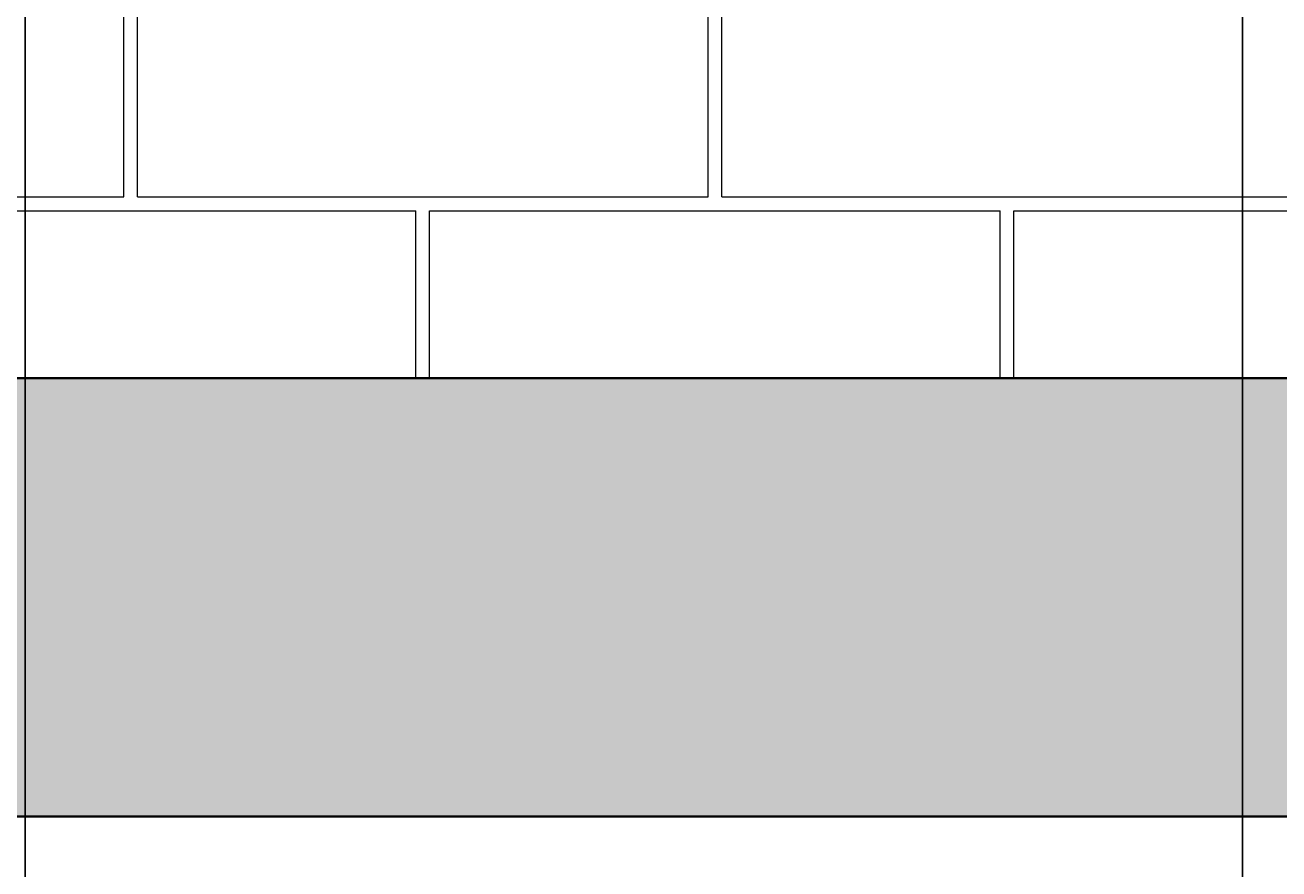
# Model space of a CAD drawing. Units: inches. Extents: x -301 to 715, y -607 to 364.
# Tile 131 of 141: x 310 to 362, y -510 to -475. Entities that reach past the tile are written whole.
import ezdxf

# ---------------------------------------------------------------- set-up
doc = ezdxf.new("R2010")
doc.units = ezdxf.units.IN
doc.header["$MEASUREMENT"] = 0
for name, color, linetype, lineweight in [('A-ANNO-DIMS', 2, 'Continuous', 18), ('A-ELEV', 220, 'Continuous', 30), ('A-ELEV-PATT', 4, 'Continuous', 13)]:
    doc.layers.add(name, color=color, linetype=linetype, lineweight=lineweight)
doc.styles.get("Standard").update_dxf_attribs({"font": 'arial.ttf'})
doc.dimstyles.get("Standard").update_dxf_attribs({"dimtxt": 0.18, "dimasz": 0.18, "dimexe": 0.18, "dimexo": 0.0625, "dimgap": 0.09, "dimtad": 0, "dimtih": 1, "dimtoh": 1, "dimdec": 1, "dimzin": 0, "dimdsep": 46, "dimlunit": 4, "dimtxsty": 'Standard', "dimcen": 0.09, "dimclrd": 3, "dimclre": 4, "dimclrt": 6, "dimadec": 0, "dimazin": 0, "dimtfac": 1, "dimtdec": 1, "dimtofl": 0, "dimtmove": 0, "dimatfit": 3, "dimfxl": 1, "dimtfill": 2, "dimtfillclr": 51, "dimtolj": 1, "dimtzin": 0, "dimarcsym": 0})

# ---------------------------------------------------------------- blocks, each defined once
blk = doc.blocks.new('*D195')
at = {"layer": 'A-ANNO-DIMS', "color": 4, "lineweight": -2, "transparency": 16777216}
for p, q in [((310.018, -441.615), (310.018, -606.789)), ((360.018, -441.615), (360.018, -606.789))]:
    blk.add_line(p, q, dxfattribs=at)
at = {"layer": 'A-ANNO-DIMS', "color": 3, "lineweight": -2, "transparency": 16777216}
for p, q in [((310.198, -606.609), (334.685, -606.609)), ((359.838, -606.609), (335.351, -606.609))]:
    blk.add_line(p, q, dxfattribs=at)
at = {"layer": 'A-ANNO-DIMS', "color": 3, "transparency": 16777216}
for points in [[(310.198, -606.579), (310.198, -606.639), (310.018, -606.609)], [(359.838, -606.579), (359.838, -606.639), (360.018, -606.609)]]:
    blk.add_solid(points, dxfattribs=at)
at = {"layer": 'Defpoints', "color": 0, "transparency": 16777216}
for p in [(310.018, -441.552), (360.018, -441.552), (360.018, -606.609)]:
    blk.add_point(p, dxfattribs=at)
at = {"layer": 'A-ANNO-DIMS', "color": 6, "transparency": 16777216, "insert": (335.018, -606.609), "char_height": 0.18, "attachment_point": 5, "bg_fill": 1, "box_fill_scale": 1.25, "bg_fill_color": 51, "bg_fill_transparency": 0}
blk.add_mtext('\\A1;4\'-2"', dxfattribs=at)
blk = doc.blocks.new('*D196')
at = {"layer": 'A-ANNO-DIMS', "color": 4, "lineweight": -2, "transparency": 16777216}
for p, q in [((360.018, -441.615), (360.018, -606.789)), ((413.018, -489.615), (413.018, -606.789))]:
    blk.add_line(p, q, dxfattribs=at)
at = {"layer": 'A-ANNO-DIMS', "color": 3, "lineweight": -2, "transparency": 16777216}
for p, q in [((360.198, -606.609), (386.185, -606.609)), ((412.838, -606.609), (386.851, -606.609))]:
    blk.add_line(p, q, dxfattribs=at)
at = {"layer": 'A-ANNO-DIMS', "color": 3, "transparency": 16777216}
for points in [[(360.198, -606.579), (360.198, -606.639), (360.018, -606.609)], [(412.838, -606.579), (412.838, -606.639), (413.018, -606.609)]]:
    blk.add_solid(points, dxfattribs=at)
at = {"layer": 'Defpoints', "color": 0, "transparency": 16777216}
for p in [(360.018, -441.552), (413.018, -489.552), (413.018, -606.609)]:
    blk.add_point(p, dxfattribs=at)
at = {"layer": 'A-ANNO-DIMS', "color": 6, "transparency": 16777216, "insert": (386.518, -606.609), "char_height": 0.18, "attachment_point": 5, "bg_fill": 1, "box_fill_scale": 1.25, "bg_fill_color": 51, "bg_fill_transparency": 0}
blk.add_mtext('\\A1;4\'-5"', dxfattribs=at)
blk = doc.blocks.new('*D200')
at = {"layer": 'A-ANNO-DIMS', "color": 4, "lineweight": -2, "transparency": 16777216}
for p, q in [((412.955, -393.552), (121.926, -393.552)), ((412.955, -489.552), (121.926, -489.552))]:
    blk.add_line(p, q, dxfattribs=at)
at = {"layer": 'A-ANNO-DIMS', "color": 3, "lineweight": -2, "transparency": 16777216}
for p, q in [((122.106, -393.732), (122.106, -441.371)), ((122.106, -489.372), (122.106, -441.734))]:
    blk.add_line(p, q, dxfattribs=at)
at = {"layer": 'A-ANNO-DIMS', "color": 3, "transparency": 16777216}
for points in [[(122.076, -393.732), (122.136, -393.732), (122.106, -393.552)], [(122.076, -489.372), (122.136, -489.372), (122.106, -489.552)]]:
    blk.add_solid(points, dxfattribs=at)
at = {"layer": 'Defpoints', "color": 0, "transparency": 16777216}
for p in [(122.106, -393.552), (413.018, -393.552), (413.018, -489.552)]:
    blk.add_point(p, dxfattribs=at)
at = {"layer": 'A-ANNO-DIMS', "color": 6, "transparency": 16777216, "insert": (122.106, -441.552), "char_height": 0.18, "attachment_point": 5, "bg_fill": 1, "box_fill_scale": 1.25, "bg_fill_color": 51, "bg_fill_transparency": 0}
blk.add_mtext('\\A1;8\'-0"', dxfattribs=at)

msp = doc.modelspace()

# ---------------------------------------------------------------- hatches: boundary and pattern name
at = {"layer": 'A-ELEV-PATT'}
h = msp.add_hatch(dxfattribs=at)
h.set_pattern_fill('AR-B816C', color=256, scale=1.5)
h.set_pattern_definition([(0, (458.621, 9.325), (12, 12), [23.4375, -0.5625]), (0, (446.621, 9.887), (12, 12), [23.4375, -0.5625]), (90, (458.621, 9.325), (-12, 12), [-12.5625, 11.4375]), (90, (458.059, 9.325), (-12, 12), [-12.5625, 11.4375])])
h.paths.add_polyline_path([(254.018, -489.552), (413.018, -489.552), (413.018, -393.552), (461.018, -393.552), (461.018, -489.552), (591.518, -489.552), (591.518, -369.552), (254.018, -369.552)])
h.paths.add_polyline_path([(310.018, -393.552), (360.018, -393.552), (360.018, -441.552), (310.018, -441.552)], flags=16)
h.paths.add_polyline_path([(315.018, -398.552), (355.018, -398.552), (355.018, -436.552), (315.018, -436.552)], flags=0)
h.paths.add_polyline_path([(496.768, -393.552), (546.768, -393.552), (546.768, -441.552), (496.768, -441.552)], flags=16)
h.paths.add_polyline_path([(501.768, -398.552), (541.768, -398.552), (541.768, -436.552), (501.768, -436.552)], flags=0)
h = msp.add_hatch(dxfattribs=at)
h.set_pattern_fill('AR-CONC', color=256, scale=2)
h.set_pattern_definition([(50, (458.621, 9.325), (14.3452, -1.25504), [1.5, -16.5]), (355, (458.621, 9.325), (-2.77503, 15.04384), [1.2, -13.2]), (100.4514, (459.817, 9.22), (11.57018, 13.7888), [1.2748, -14.02284]), (46.1842, (458.621, 13.325), (21.3448, -3.3104), [2.25, -24.75]), (96.6356, (460.4, 13.049), (18.69324, 19.4824), [1.9122, -21.0343]), (351.184, (458.62, 13.325), (18.6932, 19.4824), [1.8, -19.8]), (21, (460.621, 12.325), (11.93814, -8.05238), [1.5, -16.5]), (326, (460.621, 12.325), (4.8663, 14.503), [1.2, -13.2]), (71.4514, (461.616, 11.654), (16.80445, 6.45062), [1.2748, -14.02284]), (37.5, (458.621, 9.325), (0.243197, 6.657877), [0, -13.04, 0, -13.4, 0, -13.25]), (7.5, (458.621, 9.325), (5.26139, 7.88823), [0, -7.64, 0, -12.74, 0, -5.05]), (327.5, (454.161, 9.325), (10.67645, -0.4511), [0, -5, 0, -15.6, 0, -20.7]), (317.5, (452.161, 9.325), (11.66372, 2.0021), [0, -6.5, 0, -10.36, 0, -14.7])])
h.paths.add_polyline_path([(254.018, -489.552), (254.018, -507.552), (413.018, -507.552), (413.018, -489.552)])
h.paths.add_polyline_path([(591.518, -507.552), (591.518, -489.552), (461.018, -489.552), (461.018, -507.552)])

# ---------------------------------------------------------------- linework, layer by layer
at = {"layer": 'A-ELEV'}
for p, q in [((254.018, -489.552), (591.518, -489.552)), ((254.018, -507.552), (591.518, -507.552))]:
    msp.add_line(p, q, dxfattribs=at)
for points in [[(254.018, -369.552), (591.518, -369.552), (591.518, -489.552), (254.018, -489.552)], [(254.018, -489.552), (591.518, -489.552), (591.518, -507.552), (254.018, -507.552)]]:
    msp.add_lwpolyline(points, close=True, dxfattribs=at)

# ---------------------------------------------------------------- dimensions: what is measured, and where the dimension line sits
at = {"layer": 'A-ANNO-DIMS'}
dim = msp.add_linear_dim(base=(122.106, -393.552), p1=(413.018, -489.552), p2=(413.018, -393.552), angle=90, dimstyle='Standard', override={"dimdec": 1, "dimlfac": 1, "dimrnd": 0, "dimzin": 1, "dimdsep": 46, "dimlunit": 4, "dimfrac": 2}, dxfattribs=at)
dim.commit()
dim.dimension.update_dxf_attribs({"geometry": '*D200', "text_midpoint": (122.106, -441.552)})
for base, p1, p2, picture, middle in [((360.018, -606.609), (310.018, -441.552), (360.018, -441.552), '*D195', (335.018, -606.609)), ((413.018, -606.609), (360.018, -441.552), (413.018, -489.552), '*D196', (386.518, -606.609))]:
    dim = msp.add_linear_dim(base=base, p1=p1, p2=p2, dimstyle='Standard', override={"dimdec": 1, "dimlfac": 1, "dimrnd": 0, "dimzin": 1, "dimdsep": 46, "dimlunit": 4, "dimfrac": 2}, dxfattribs=at)
    dim.commit()
    dim.dimension.update_dxf_attribs({"geometry": picture, "text_midpoint": middle})

doc.saveas('drawing.dxf')
